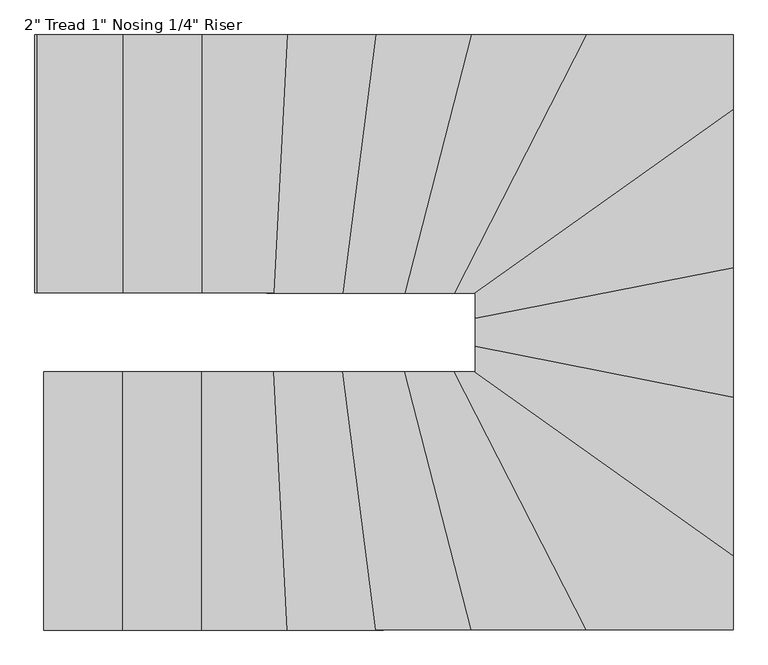
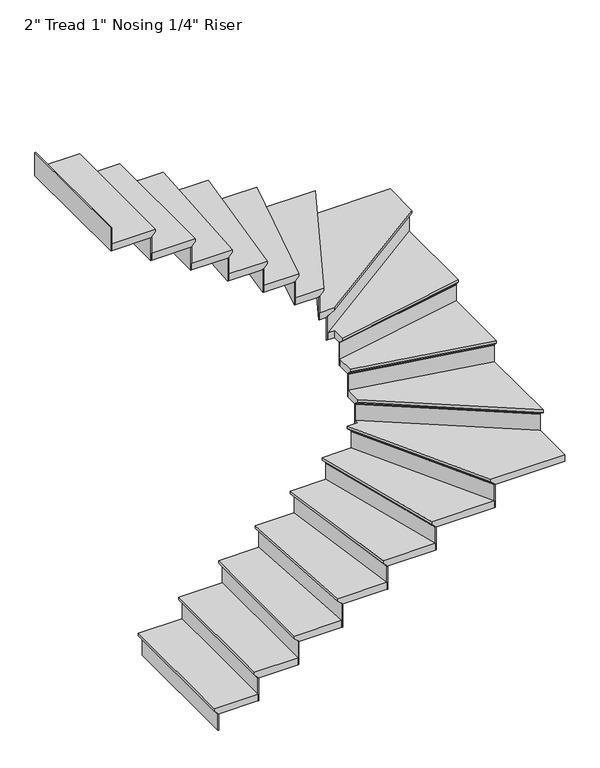
"""IFC4 building model written with IfcOpenShell, lengths in millimetres: stair flight geometry."""

from ifc_helpers import new_model, si_unit, origin, place, context, project, spatial, faceted_brep, source, transform, mapped, element, save


def stair_flight_916a27e3(model_context):
    return source(origin(), model_context, "Body", "Brep", [
        faceted_brep([(531.7538115, -7565.2090409, 12951.8833333), (531.7538115, -7565.2090409, 12970.9333333), (531.7538115, -6650.8090409, 12970.9333333), (531.7538115, -6650.8090409, 12951.8833333), (557.1538115, -7565.2090409, 12926.4833333), (557.1538115, -6650.8090409, 12926.4833333), (836.5538115, -7565.2090409, 12970.9333333), (836.5538115, -6650.8090409, 12970.9333333), (557.1538115, -6650.8090409, 12920.1333333), (836.5538115, -6650.8090409, 12920.1333333), (836.5538115, -7565.2090409, 12920.1333333), (557.1538115, -7565.2090409, 12920.1333333)], [[[0, 1, 2, 3]], [[4, 0, 3, 5]], [[2, 1, 6, 7]], [[8, 9, 10, 11]], [[2, 7, 9, 8, 5, 3]], [[8, 11, 4, 5]], [[6, 1, 0, 4, 11, 10]], [[7, 6, 10, 9]]]),
        faceted_brep([(557.1538115, -7565.2090409, 12920.1333333), (557.1538115, -7565.2090409, 12801.6), (563.5038115, -7565.2090409, 12801.6), (563.5038115, -7565.2090409, 12920.1333333), (557.1538115, -6650.8090409, 12920.1333333), (563.5038115, -6650.8090409, 12920.1333333), (563.5038115, -6650.8090409, 12801.6), (557.1538115, -6650.8090409, 12801.6)], [[[0, 1, 2, 3]], [[4, 5, 6, 7]], [[1, 0, 4, 7]], [[2, 1, 7, 6]], [[3, 2, 6, 5]], [[0, 3, 5, 4]]]),
        faceted_brep([(836.5538115, -7565.2090409, 13089.4666667), (836.5538115, -7565.2090409, 12920.1333333), (842.9038115, -7565.2090409, 12920.1333333), (842.9038115, -7565.2090409, 13089.4666667), (836.5538115, -6650.8090409, 13089.4666667), (842.9038115, -6650.8090409, 13089.4666667), (842.9038115, -6650.8090409, 12920.1333333), (836.5538115, -6650.8090409, 12920.1333333)], [[[0, 1, 2, 3]], [[4, 5, 6, 7]], [[1, 0, 4, 7]], [[2, 1, 7, 6]], [[3, 2, 6, 5]], [[0, 3, 5, 4]]]),
        faceted_brep([(811.1538115, -6650.8090409, 13140.2666667), (811.1538115, -7565.2090409, 13140.2666667), (1115.9538115, -7565.2090409, 13140.2666667), (1115.9538115, -6650.8090409, 13140.2666667), (836.5538115, -6650.8090409, 13089.4666667), (1115.9538115, -6650.8090409, 13089.4666667), (1115.9538115, -7565.2090409, 13089.4666667), (836.5538115, -7565.2090409, 13089.4666667), (836.5538115, -6650.8090409, 13095.8166667), (811.1538115, -6650.8090409, 13121.2166667), (836.5538115, -7565.2090409, 13095.8166667), (811.1538115, -7565.2090409, 13121.2166667)], [[[0, 1, 2, 3]], [[4, 5, 6, 7]], [[0, 3, 5, 4, 8, 9]], [[4, 7, 10, 8]], [[2, 1, 11, 10, 7, 6]], [[3, 2, 6, 5]], [[11, 1, 0, 9]], [[10, 11, 9, 8]]]),
        faceted_brep([(1115.9538115, -7565.2090409, 13258.8), (1115.9538115, -7565.2090409, 13089.4666667), (1122.3038115, -7565.2090409, 13089.4666667), (1122.3038115, -7565.2090409, 13258.8), (1115.9538115, -6650.8090409, 13258.8), (1122.3038115, -6650.8090409, 13258.8), (1122.3038115, -6650.8090409, 13089.4666667), (1115.9538115, -6650.8090409, 13089.4666667)], [[[0, 1, 2, 3]], [[4, 5, 6, 7]], [[1, 0, 4, 7]], [[2, 1, 7, 6]], [[3, 2, 6, 5]], [[0, 3, 5, 4]]]),
        faceted_brep([(1090.5538115, -6650.8090409, 13309.6), (1090.5538115, -7565.2090409, 13309.6), (1419.1552434, -7565.2090409, 13309.6), (1371.620973, -6650.8090409, 13309.6), (1115.9538115, -6650.8090409, 13258.8), (1371.620973, -6650.8090409, 13258.8), (1419.1552434, -7565.2090409, 13258.8), (1115.9538115, -7565.2090409, 13258.8), (1115.9538115, -6650.8090409, 13265.15), (1090.5538115, -6650.8090409, 13290.55), (1115.9538115, -7565.2090409, 13265.15), (1090.5538115, -7565.2090409, 13290.55)], [[[0, 1, 2, 3]], [[4, 5, 6, 7]], [[0, 3, 5, 4, 8, 9]], [[4, 7, 10, 8]], [[2, 1, 11, 10, 7, 6]], [[3, 2, 6, 5]], [[11, 1, 0, 9]], [[10, 11, 9, 8]]]),
        faceted_brep([(1419.1552434, -7565.2090409, 13428.1333333), (1419.1552434, -7565.2090409, 13258.8), (1425.5138176, -7565.2090409, 13258.8), (1425.5138176, -7565.2090409, 13428.1333333), (1371.620973, -6650.8090409, 13428.1333333), (1377.9795471, -6650.8090409, 13428.1333333), (1377.9795471, -6650.8090409, 13258.8), (1371.620973, -6650.8090409, 13258.8)], [[[0, 1, 2, 3]], [[4, 5, 6, 7]], [[1, 0, 4, 7]], [[2, 1, 7, 6]], [[3, 2, 6, 5]], [[0, 3, 5, 4]]]),
        faceted_brep([(1346.1866763, -6650.8090409, 13478.9333333), (1393.7209467, -7565.2090409, 13478.9333333), (1734.1437245, -7565.2090409, 13478.9333333), (1615.7876728, -6650.8090409, 13478.9333333), (1371.620973, -6650.8090409, 13428.1333333), (1615.7876728, -6650.8090409, 13428.1333333), (1734.1437245, -7565.2090409, 13428.1333333), (1419.1552434, -7565.2090409, 13428.1333333), (1371.620973, -6650.8090409, 13434.4833333), (1346.1866763, -6650.8090409, 13459.8833333), (1419.1552434, -7565.2090409, 13434.4833333), (1393.7209467, -7565.2090409, 13459.8833333)], [[[0, 1, 2, 3]], [[4, 5, 6, 7]], [[0, 3, 5, 4, 8, 9]], [[4, 7, 10, 8]], [[2, 1, 11, 10, 7, 6]], [[3, 2, 6, 5]], [[11, 1, 0, 9]], [[10, 11, 9, 8]]]),
        faceted_brep([(1734.1437245, -7565.2090409, 13597.4666667), (1734.1437245, -7565.2090409, 13428.1333333), (1740.5466962, -7565.2090409, 13428.1333333), (1740.5466962, -7565.2090409, 13597.4666667), (1615.7876728, -6650.8090409, 13597.4666667), (1622.1906446, -6650.8090409, 13597.4666667), (1622.1906446, -6650.8090409, 13428.1333333), (1615.7876728, -6650.8090409, 13428.1333333)], [[[0, 1, 2, 3]], [[4, 5, 6, 7]], [[1, 0, 4, 7]], [[2, 1, 7, 6]], [[3, 2, 6, 5]], [[0, 3, 5, 4]]]),
        faceted_brep([(1590.1757857, -6650.8090409, 13648.2666667), (1708.5318374, -7565.2090409, 13648.2666667), (2072.5453427, -7565.2090409, 13648.2666667), (1837.4148953, -6650.8090409, 13648.2666667), (1615.7876728, -6650.8090409, 13597.4666667), (1837.4148953, -6650.8090409, 13597.4666667), (2072.5453427, -7565.2090409, 13597.4666667), (1734.1437245, -7565.2090409, 13597.4666667), (1615.7876728, -6650.8090409, 13603.8166667), (1590.1757857, -6650.8090409, 13629.2166667), (1734.1437245, -7565.2090409, 13603.8166667), (1708.5318374, -7565.2090409, 13629.2166667)], [[[0, 1, 2, 3]], [[4, 5, 6, 7]], [[0, 3, 5, 4, 8, 9]], [[4, 7, 10, 8]], [[2, 1, 11, 10, 7, 6]], [[3, 2, 6, 5]], [[11, 1, 0, 9]], [[10, 11, 9, 8]]]),
        faceted_brep([(2072.5453427, -7565.2090409, 13766.8), (2072.5453427, -7565.2090409, 13597.4666667), (2079.1019196, -7565.2090409, 13597.4666667), (2079.1019196, -7565.2090409, 13766.8), (1837.4148953, -6650.8090409, 13766.8), (1843.9714722, -6650.8090409, 13766.8), (1843.9714722, -6650.8090409, 13597.4666667), (1837.4148953, -6650.8090409, 13597.4666667)], [[[0, 1, 2, 3]], [[4, 5, 6, 7]], [[1, 0, 4, 7]], [[2, 1, 7, 6]], [[3, 2, 6, 5]], [[0, 3, 5, 4]]]),
        faceted_brep([(1811.1885878, -6650.8090409, 13817.6), (2046.3190352, -7565.2090409, 13817.6), (2482.5861527, -7565.2090409, 13817.6), (2013.7615314, -6650.8090409, 13817.6), (1837.4148953, -6650.8090409, 13766.8), (2013.7615314, -6650.8090409, 13766.8), (2482.5861527, -7565.2090409, 13766.8), (2072.5453427, -7565.2090409, 13766.8), (1837.4148953, -6650.8090409, 13773.15), (1811.1885878, -6650.8090409, 13798.55), (2072.5453427, -7565.2090409, 13773.15), (2046.3190352, -7565.2090409, 13798.55)], [[[0, 1, 2, 3]], [[4, 5, 6, 7]], [[0, 3, 5, 4, 8, 9]], [[4, 7, 10, 8]], [[2, 1, 11, 10, 7, 6]], [[3, 2, 6, 5]], [[11, 1, 0, 9]], [[10, 11, 9, 8]]]),
        faceted_brep([(2482.5861527, -7565.2090409, 13936.1333333), (2482.5861527, -7565.2090409, 13766.8), (2489.7221358, -7565.2090409, 13766.8), (2489.7221358, -7565.2090409, 13936.1333333), (2013.7615314, -6650.8090409, 13936.1333333), (2020.8975145, -6650.8090409, 13936.1333333), (2020.8975145, -6650.8090409, 13766.8), (2013.7615314, -6650.8090409, 13766.8)], [[[0, 1, 2, 3]], [[4, 5, 6, 7]], [[1, 0, 4, 7]], [[2, 1, 7, 6]], [[3, 2, 6, 5]], [[0, 3, 5, 4]]]),
        faceted_brep([(2059.4855034, -6621.253958, 13986.9333333), (2059.4855034, -6650.8090409, 13986.9333333), (1985.2175988, -6650.8090409, 13986.9333333), (2454.0422202, -7565.2090409, 13986.9333333), (2973.8855034, -7565.2090409, 13986.9333333), (2973.8855034, -7271.5279072, 13986.9333333), (2059.4855034, -6650.8090409, 13936.1333333), (2059.4855034, -6621.253958, 13936.1333333), (2973.8855034, -7271.5279072, 13936.1333333), (2973.8855034, -7565.2090409, 13936.1333333), (2482.5861527, -7565.2090409, 13936.1333333), (2013.7615314, -6650.8090409, 13936.1333333), (2013.7615314, -6650.8090409, 13942.4833333), (1985.2175988, -6650.8090409, 13967.8833333), (2482.5861527, -7565.2090409, 13942.4833333), (2454.0422202, -7565.2090409, 13967.8833333)], [[[0, 1, 2, 3, 4, 5]], [[6, 7, 8, 9, 10, 11]], [[1, 0, 7, 6]], [[2, 1, 6, 11, 12, 13]], [[11, 10, 14, 12]], [[4, 3, 15, 14, 10, 9]], [[5, 4, 9, 8]], [[0, 5, 8, 7]], [[15, 3, 2, 13]], [[14, 15, 13, 12]]]),
        faceted_brep([(2973.8855034, -7271.5279072, 14105.4666667), (2973.8855034, -7271.5279072, 13936.1333333), (2973.8855034, -7263.7359324, 13936.1333333), (2973.8855034, -7263.7359324, 14105.4666667), (2059.4855034, -6621.253958, 14105.4666667), (2059.4855034, -6613.4619832, 14105.4666667), (2059.4855034, -6613.4619832, 13936.1333333), (2059.4855034, -6621.253958, 13936.1333333)], [[[0, 1, 2, 3]], [[4, 5, 6, 7]], [[1, 0, 4, 7]], [[2, 1, 7, 6]], [[3, 2, 6, 5]], [[0, 3, 5, 4]]]),
        faceted_brep([(2059.4855034, -6652.4218572, 14156.2666667), (2973.8855034, -7302.6958063, 14156.2666667), (2973.8855034, -6715.0407273, 14156.2666667), (2059.4855034, -6534.7998709, 14156.2666667), (2059.4855034, -6621.253958, 14105.4666667), (2059.4855034, -6534.7998709, 14105.4666667), (2973.8855034, -6715.0407273, 14105.4666667), (2973.8855034, -7271.5279072, 14105.4666667), (2059.4855034, -6621.253958, 14111.8166667), (2059.4855034, -6652.4218572, 14137.2166667), (2973.8855034, -7271.5279072, 14111.8166667), (2973.8855034, -7302.6958063, 14137.2166667)], [[[0, 1, 2, 3]], [[4, 5, 6, 7]], [[0, 3, 5, 4, 8, 9]], [[4, 7, 10, 8]], [[3, 2, 6, 5]], [[11, 1, 0, 9]], [[10, 11, 9, 8]], [[2, 1, 11, 10, 7, 6]]]),
        faceted_brep([(2973.8855034, -6715.0407273, 14274.8), (2973.8855034, -6715.0407273, 14105.4666667), (2973.8855034, -6708.5685418, 14105.4666667), (2973.8855034, -6708.5685418, 14274.8), (2059.4855034, -6534.7998709, 14274.8), (2059.4855034, -6528.3276855, 14274.8), (2059.4855034, -6528.3276855, 14105.4666667), (2059.4855034, -6534.7998709, 14105.4666667)], [[[0, 1, 2, 3]], [[4, 5, 6, 7]], [[1, 0, 4, 7]], [[2, 1, 7, 6]], [[3, 2, 6, 5]], [[0, 3, 5, 4]]]),
        faceted_brep([(2059.4855034, -6560.6886127, 14325.6), (2973.8855034, -6740.929469, 14325.6), (2973.8855034, -6255.3998709, 14325.6), (2059.4855034, -6435.6407273, 14325.6), (2059.4855034, -6534.7998709, 14274.8), (2059.4855034, -6435.6407273, 14274.8), (2973.8855034, -6255.3998709, 14274.8), (2973.8855034, -6715.0407273, 14274.8), (2059.4855034, -6534.7998709, 14281.15), (2059.4855034, -6560.6886127, 14306.55), (2973.8855034, -6715.0407273, 14281.15), (2973.8855034, -6740.929469, 14306.55)], [[[0, 1, 2, 3]], [[4, 5, 6, 7]], [[0, 3, 5, 4, 8, 9]], [[4, 7, 10, 8]], [[2, 1, 11, 10, 7, 6]], [[3, 2, 6, 5]], [[11, 1, 0, 9]], [[10, 11, 9, 8]]]),
        faceted_brep([(2973.8855034, -6255.3998709, 14444.1333333), (2973.8855034, -6255.3998709, 14274.8), (2973.8855034, -6248.9276855, 14274.8), (2973.8855034, -6248.9276855, 14444.1333333), (2059.4855034, -6435.6407273, 14444.1333333), (2059.4855034, -6429.1685418, 14444.1333333), (2059.4855034, -6429.1685418, 14274.8), (2059.4855034, -6435.6407273, 14274.8)], [[[0, 1, 2, 3]], [[4, 5, 6, 7]], [[1, 0, 4, 7]], [[2, 1, 7, 6]], [[3, 2, 6, 5]], [[0, 3, 5, 4]]]),
        faceted_brep([(2013.3900289, -6371.4090409, 14494.9333333), (2059.4855034, -6371.4090409, 14494.9333333), (2059.4855034, -6461.529469, 14494.9333333), (2973.8855034, -6281.2886127, 14494.9333333), (2973.8855034, -5688.3543762, 14494.9333333), (2059.4855034, -6371.4090409, 14444.1333333), (2013.3900289, -6371.4090409, 14444.1333333), (2973.8855034, -5688.3543762, 14444.1333333), (2973.8855034, -6255.3998709, 14444.1333333), (2059.4855034, -6435.6407273, 14444.1333333), (2973.8855034, -6255.3998709, 14450.4833333), (2059.4855034, -6435.6407273, 14450.4833333), (2973.8855034, -6281.2886127, 14475.8833333), (2059.4855034, -6461.529469, 14475.8833333)], [[[0, 1, 2, 3, 4]], [[5, 6, 7, 8, 9]], [[1, 0, 6, 5]], [[9, 8, 10, 11]], [[4, 3, 12, 10, 8, 7]], [[0, 4, 7, 6]], [[12, 3, 2, 13]], [[10, 12, 13, 11]], [[2, 1, 5, 9, 11, 13]]]),
        faceted_brep([(2973.8855034, -5688.3543762, 14613.4666667), (2973.8855034, -5688.3543762, 14444.1333333), (2973.8855034, -5680.5624014, 14444.1333333), (2973.8855034, -5680.5624014, 14613.4666667), (2013.3900289, -6371.4090409, 14613.4666667), (2002.4331364, -6371.4090409, 14613.4666667), (2002.4331364, -6371.4090409, 14444.1333333), (2013.3900289, -6371.4090409, 14444.1333333)], [[[0, 1, 2, 3]], [[4, 5, 6, 7]], [[1, 0, 4, 7]], [[2, 1, 7, 6]], [[3, 2, 6, 5]], [[0, 3, 5, 4]]]),
        faceted_brep([(2057.2175988, -6371.4090409, 14664.2666667), (2973.8855034, -5719.5222754, 14664.2666667), (2973.8855034, -5457.0090409, 14664.2666667), (2425.4982876, -5457.0090409, 14664.2666667), (1956.6736663, -6371.4090409, 14664.2666667), (2013.3900289, -6371.4090409, 14613.4666667), (1956.6736663, -6371.4090409, 14613.4666667), (2425.4982876, -5457.0090409, 14613.4666667), (2973.8855034, -5457.0090409, 14613.4666667), (2973.8855034, -5688.3543762, 14613.4666667), (2013.3900289, -6371.4090409, 14619.8166667), (2057.2175988, -6371.4090409, 14645.2166667), (2973.8855034, -5688.3543762, 14619.8166667), (2973.8855034, -5719.5222754, 14645.2166667)], [[[0, 1, 2, 3, 4]], [[5, 6, 7, 8, 9]], [[0, 4, 6, 5, 10, 11]], [[5, 9, 12, 10]], [[2, 1, 13, 12, 9, 8]], [[4, 3, 7, 6]], [[13, 1, 0, 11]], [[12, 13, 11, 10]], [[3, 2, 8, 7]]]),
        faceted_brep([(2425.4982876, -5457.0090409, 14782.8), (2425.4982876, -5457.0090409, 14613.4666667), (2418.3623045, -5457.0090409, 14613.4666667), (2418.3623045, -5457.0090409, 14782.8), (1956.6736663, -6371.4090409, 14782.8), (1949.5376832, -6371.4090409, 14782.8), (1949.5376832, -6371.4090409, 14613.4666667), (1956.6736663, -6371.4090409, 14613.4666667)], [[[0, 1, 2, 3]], [[4, 5, 6, 7]], [[1, 0, 4, 7]], [[2, 1, 7, 6]], [[3, 2, 6, 5]], [[0, 3, 5, 4]]]),
        faceted_brep([(1985.2175988, -6371.4090409, 14833.6), (2454.0422202, -5457.0090409, 14833.6), (2020.0927278, -5457.0090409, 14833.6), (1784.9622804, -6371.4090409, 14833.6), (1956.6736663, -6371.4090409, 14782.8), (1784.9622804, -6371.4090409, 14782.8), (2020.0927278, -5457.0090409, 14782.8), (2425.4982876, -5457.0090409, 14782.8), (1956.6736663, -6371.4090409, 14789.15), (1985.2175988, -6371.4090409, 14814.55), (2425.4982876, -5457.0090409, 14789.15), (2454.0422202, -5457.0090409, 14814.55)], [[[0, 1, 2, 3]], [[4, 5, 6, 7]], [[0, 3, 5, 4, 8, 9]], [[4, 7, 10, 8]], [[2, 1, 11, 10, 7, 6]], [[3, 2, 6, 5]], [[11, 1, 0, 9]], [[10, 11, 9, 8]]]),
        faceted_brep([(2020.0927278, -5457.0090409, 14952.1333333), (2020.0927278, -5457.0090409, 14782.8), (2013.5361509, -5457.0090409, 14782.8), (2013.5361509, -5457.0090409, 14952.1333333), (1784.9622804, -6371.4090409, 14952.1333333), (1778.4057035, -6371.4090409, 14952.1333333), (1778.4057035, -6371.4090409, 14782.8), (1784.9622804, -6371.4090409, 14782.8)], [[[0, 1, 2, 3]], [[4, 5, 6, 7]], [[1, 0, 4, 7]], [[2, 1, 7, 6]], [[3, 2, 6, 5]], [[0, 3, 5, 4]]]),
        faceted_brep([(1811.1885878, -6371.4090409, 15002.9333333), (2046.3190352, -5457.0090409, 15002.9333333), (1682.9199502, -5457.0090409, 15002.9333333), (1564.5638986, -6371.4090409, 15002.9333333), (1784.9622804, -6371.4090409, 14952.1333333), (1564.5638986, -6371.4090409, 14952.1333333), (1682.9199502, -5457.0090409, 14952.1333333), (2020.0927278, -5457.0090409, 14952.1333333), (1784.9622804, -6371.4090409, 14958.4833333), (1811.1885878, -6371.4090409, 14983.8833333), (2020.0927278, -5457.0090409, 14958.4833333), (2046.3190352, -5457.0090409, 14983.8833333)], [[[0, 1, 2, 3]], [[4, 5, 6, 7]], [[0, 3, 5, 4, 8, 9]], [[4, 7, 10, 8]], [[2, 1, 11, 10, 7, 6]], [[3, 2, 6, 5]], [[11, 1, 0, 9]], [[10, 11, 9, 8]]]),
        faceted_brep([(1682.9199502, -5457.0090409, 15121.4666667), (1682.9199502, -5457.0090409, 14952.1333333), (1676.5169785, -5457.0090409, 14952.1333333), (1676.5169785, -5457.0090409, 15121.4666667), (1564.5638986, -6371.4090409, 15121.4666667), (1558.1609268, -6371.4090409, 15121.4666667), (1558.1609268, -6371.4090409, 14952.1333333), (1564.5638986, -6371.4090409, 14952.1333333)], [[[0, 1, 2, 3]], [[4, 5, 6, 7]], [[1, 0, 4, 7]], [[2, 1, 7, 6]], [[3, 2, 6, 5]], [[0, 3, 5, 4]]]),
        faceted_brep([(1590.1757857, -6371.4090409, 15172.2666667), (1708.5318374, -5457.0090409, 15172.2666667), (1368.2866501, -5457.0090409, 15172.2666667), (1320.7523797, -6371.4090409, 15172.2666667), (1564.5638986, -6371.4090409, 15121.4666667), (1320.7523797, -6371.4090409, 15121.4666667), (1368.2866501, -5457.0090409, 15121.4666667), (1682.9199502, -5457.0090409, 15121.4666667), (1564.5638986, -6371.4090409, 15127.8166667), (1590.1757857, -6371.4090409, 15153.2166667), (1682.9199502, -5457.0090409, 15127.8166667), (1708.5318374, -5457.0090409, 15153.2166667)], [[[0, 1, 2, 3]], [[4, 5, 6, 7]], [[0, 3, 5, 4, 8, 9]], [[4, 7, 10, 8]], [[2, 1, 11, 10, 7, 6]], [[3, 2, 6, 5]], [[11, 1, 0, 9]], [[10, 11, 9, 8]]]),
        faceted_brep([(1368.2866501, -5457.0090409, 15290.8), (1368.2866501, -5457.0090409, 15121.4666667), (1361.9280759, -5457.0090409, 15121.4666667), (1361.9280759, -5457.0090409, 15290.8), (1320.7523797, -6371.4090409, 15290.8), (1314.3938055, -6371.4090409, 15290.8), (1314.3938055, -6371.4090409, 15121.4666667), (1320.7523797, -6371.4090409, 15121.4666667)], [[[0, 1, 2, 3]], [[4, 5, 6, 7]], [[1, 0, 4, 7]], [[2, 1, 7, 6]], [[3, 2, 6, 5]], [[0, 3, 5, 4]]]),
        faceted_brep([(1346.1866763, -6371.4090409, 15341.6), (1393.7209467, -5457.0090409, 15341.6), (1065.1538115, -5457.0090409, 15341.6), (1065.1538115, -6371.4090409, 15341.6), (1320.7523797, -6371.4090409, 15290.8), (1065.1538115, -6371.4090409, 15290.8), (1065.1538115, -5457.0090409, 15290.8), (1368.2866501, -5457.0090409, 15290.8), (1320.7523797, -6371.4090409, 15297.15), (1346.1866763, -6371.4090409, 15322.55), (1368.2866501, -5457.0090409, 15297.15), (1393.7209467, -5457.0090409, 15322.55)], [[[0, 1, 2, 3]], [[4, 5, 6, 7]], [[0, 3, 5, 4, 8, 9]], [[4, 7, 10, 8]], [[2, 1, 11, 10, 7, 6]], [[3, 2, 6, 5]], [[11, 1, 0, 9]], [[10, 11, 9, 8]]]),
        faceted_brep([(1065.1538115, -5457.0090409, 15460.1333333), (1065.1538115, -5457.0090409, 15290.8), (1058.8038115, -5457.0090409, 15290.8), (1058.8038115, -5457.0090409, 15460.1333333), (1065.1538115, -6371.4090409, 15460.1333333), (1058.8038115, -6371.4090409, 15460.1333333), (1058.8038115, -6371.4090409, 15290.8), (1065.1538115, -6371.4090409, 15290.8)], [[[0, 1, 2, 3]], [[4, 5, 6, 7]], [[1, 0, 4, 7]], [[2, 1, 7, 6]], [[3, 2, 6, 5]], [[0, 3, 5, 4]]]),
        faceted_brep([(1090.5538115, -6371.4090409, 15510.9333333), (1090.5538115, -5457.0090409, 15510.9333333), (785.7538115, -5457.0090409, 15510.9333333), (785.7538115, -6371.4090409, 15510.9333333), (1065.1538115, -6371.4090409, 15460.1333333), (785.7538115, -6371.4090409, 15460.1333333), (785.7538115, -5457.0090409, 15460.1333333), (1065.1538115, -5457.0090409, 15460.1333333), (1065.1538115, -6371.4090409, 15466.4833333), (1090.5538115, -6371.4090409, 15491.8833333), (1065.1538115, -5457.0090409, 15466.4833333), (1090.5538115, -5457.0090409, 15491.8833333)], [[[0, 1, 2, 3]], [[4, 5, 6, 7]], [[0, 3, 5, 4, 8, 9]], [[4, 7, 10, 8]], [[2, 1, 11, 10, 7, 6]], [[3, 2, 6, 5]], [[11, 1, 0, 9]], [[10, 11, 9, 8]]]),
        faceted_brep([(785.7538115, -5457.0090409, 15629.4666667), (785.7538115, -5457.0090409, 15460.1333333), (779.4038115, -5457.0090409, 15460.1333333), (779.4038115, -5457.0090409, 15629.4666667), (785.7538115, -6371.4090409, 15629.4666667), (779.4038115, -6371.4090409, 15629.4666667), (779.4038115, -6371.4090409, 15460.1333333), (785.7538115, -6371.4090409, 15460.1333333)], [[[0, 1, 2, 3]], [[4, 5, 6, 7]], [[1, 0, 4, 7]], [[2, 1, 7, 6]], [[3, 2, 6, 5]], [[0, 3, 5, 4]]]),
        faceted_brep([(506.3538115, -5457.0090409, 15798.8), (506.3538115, -5457.0090409, 15629.4666667), (500.0038115, -5457.0090409, 15629.4666667), (500.0038115, -5457.0090409, 15798.8), (506.3538115, -6371.4090409, 15798.8), (500.0038115, -6371.4090409, 15798.8), (500.0038115, -6371.4090409, 15629.4666667), (506.3538115, -6371.4090409, 15629.4666667)], [[[0, 1, 2, 3]], [[4, 5, 6, 7]], [[1, 0, 4, 7]], [[2, 1, 7, 6]], [[3, 2, 6, 5]], [[0, 3, 5, 4]]]),
        faceted_brep([(811.1538115, -6371.4090409, 15680.2666667), (811.1538115, -5457.0090409, 15680.2666667), (506.3538115, -5457.0090409, 15680.2666667), (506.3538115, -6371.4090409, 15680.2666667), (785.7538115, -6371.4090409, 15629.4666667), (506.3538115, -6371.4090409, 15629.4666667), (506.3538115, -5457.0090409, 15629.4666667), (785.7538115, -5457.0090409, 15629.4666667), (785.7538115, -6371.4090409, 15635.8166667), (811.1538115, -6371.4090409, 15661.2166667), (785.7538115, -5457.0090409, 15635.8166667), (811.1538115, -5457.0090409, 15661.2166667)], [[[0, 1, 2, 3]], [[4, 5, 6, 7]], [[0, 3, 5, 4, 8, 9]], [[4, 7, 10, 8]], [[2, 1, 11, 10, 7, 6]], [[3, 2, 6, 5]], [[11, 1, 0, 9]], [[10, 11, 9, 8]]]),
    ])


if __name__ == "__main__":
    model = new_model("IFC4")
    model_context = context("Model", 3, world=origin())
    ifc_project = project(units=[si_unit("LENGTHUNIT", "METRE", prefix="MILLI")], contexts=[model_context])
    site = spatial("IfcSite", under=ifc_project)
    building = spatial("IfcBuilding", under=site)
    placement = place(None, origin())
    stair_flight_shape = stair_flight_916a27e3(model_context)
    element("IfcStairFlight", 1, ObjectType="2\" Tread 1\" Nosing 1/4\" Riser", at=placement, inside=building, context=model_context, shape_type="MappedRepresentation", body=[
        mapped(stair_flight_shape, transform((0.0, 0.0, 0.0), x_axis=(1.0, 0.0, 0.0), y_axis=(0.0, 1.0, 0.0), z_axis=(0.0, 0.0, 1.0))),
    ])
    save(model, "model.ifc")
